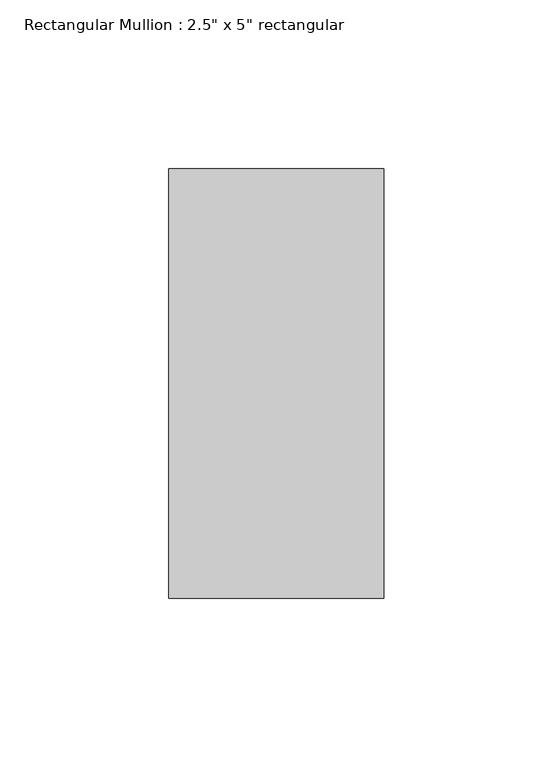
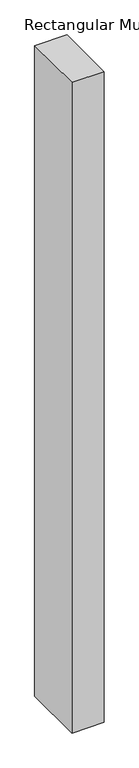
"""IFC4 building model written with IfcOpenShell, lengths in millimetres: member geometry."""

from ifc_helpers import new_model, si_unit, frame, origin, place, context, project, spatial, polyline, outline, extrude, source, transform, mapped, element, save


def member_0d0414c4(model_context):
    return source(origin(), model_context, "Body", "SweptSolid", [
        extrude(outline(polyline([(0.0, 63.5), (0.0, -63.5), (-63.5, -63.5), (-63.5, 63.5), (0.0, 63.5)])), frame((0.0, 0.0, -1358.9), z_axis=(0.0, 0.0, 1.0), x_axis=(1.0, 0.0, 0.0)), (0.0, 0.0, 1.0), 1358.9),
    ])


if __name__ == "__main__":
    model = new_model("IFC4")
    model_context = context("Model", 3, world=origin())
    ifc_project = project(units=[si_unit("LENGTHUNIT", "METRE", prefix="MILLI")], contexts=[model_context])
    site = spatial("IfcSite", under=ifc_project)
    building = spatial("IfcBuilding", under=site)
    placement = place(None, origin())
    member_shape = member_0d0414c4(model_context)
    element("IfcMember", 1, ObjectType="Rectangular Mullion : 2.5\" x 5\" rectangular", at=placement, inside=building, context=model_context, shape_type="MappedRepresentation", body=[
        mapped(member_shape, transform((0.0, 0.0, 0.0), x_axis=(1.0, 0.0, 0.0), y_axis=(0.0, 1.0, 0.0), z_axis=(0.0, 0.0, 1.0))),
    ])
    save(model, "model.ifc")

# Revit data of these elements
# Type "Rectangular Mullion : 2.5\" x 5\" rectangular"
#   built-in parameter 1007304 = 0.416667 (stored number, unit not read)
#   built-in parameter 1007301 = 0.104167 (stored number, unit not read)
#   built-in parameter 1007300 = 0.104167 (stored number, unit not read)
# Element 1 (IfcMember, "Rectangular Mullion : 2.5\" x 5\" rectangular")
#   Materials on its faces: "Aluminum"
# Materials
#   "Aluminum": class "Metal", colour RGB 247 247 247, transparency 0, Description = "Aluminum 6061", Cost = 0
